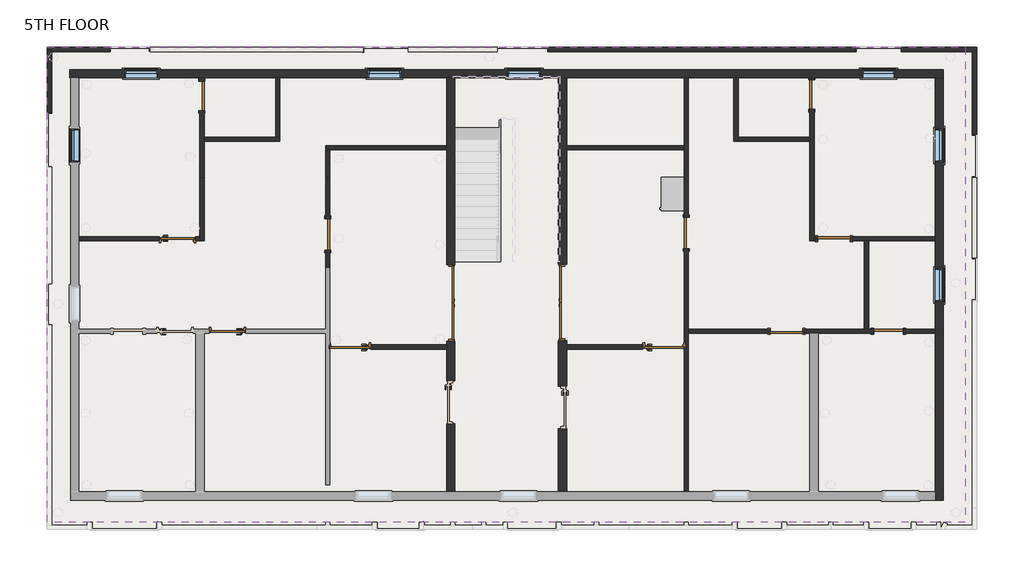
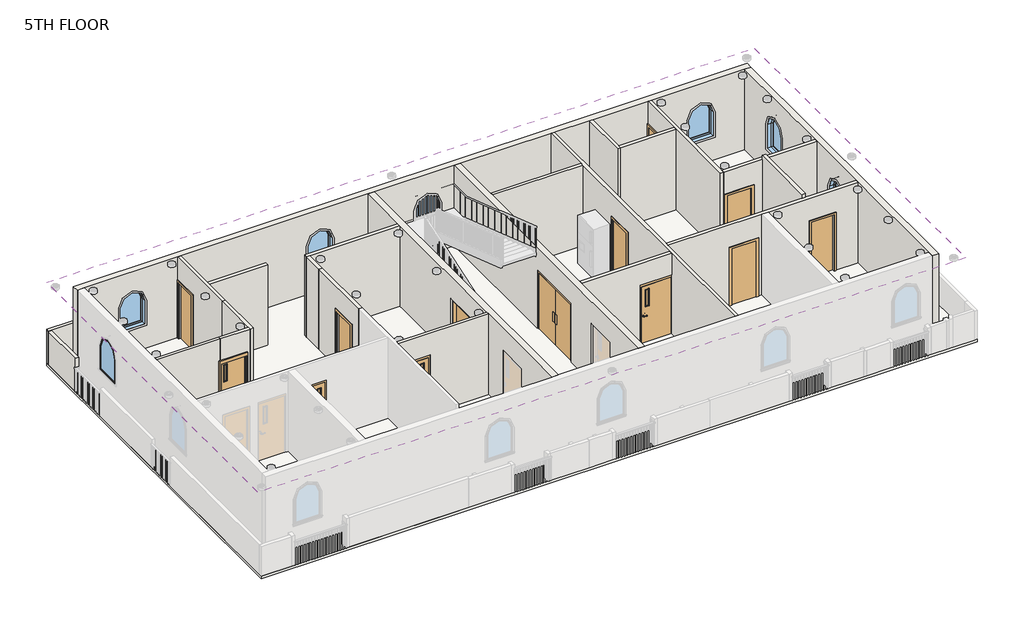
# One storey, part 2 of 7: 32 walls, 13 doors, 7 windows, 2 slabs, 1 covering.
"""IFC4 building model written with IfcOpenShell, lengths in millimetres."""

from ifc_helpers import new_model, si_unit, frame, origin, place, context, project, spatial, polyline, circle_curve, outline, extrude, faceted_brep, transform, mapped, element, save
from ifc_brep_helpers import plane_surface, revolved_surface, advanced_brep
from components import door_2c854dd0, door_cf1f2706, door_4f5842df, door_passage_single_vision_lite_3_x7_440dd290, door_70e57c00, door_700d3439, door_8cb1b8a7, door_38851409, door_d141acb4, window_fixed_round_top_3_x_4_dee2be1c

model = new_model("IFC4")

# Units and contexts
model_context = context("Model", 3, world=origin())
ifc_project = project(units=[si_unit("LENGTHUNIT", "METRE", prefix="MILLI")], contexts=[model_context])

# Site, building, storey
site = spatial("IfcSite", under=ifc_project)
building = spatial("IfcBuilding", under=site)
storey = spatial("IfcBuildingStorey", under=building, Name="5TH FLOOR", Elevation=16002.0)

# Covering
placement = place(None, origin())
element("IfcCovering", 1, ObjectType="2' x 4' ACT System", at=placement, inside=storey, context=model_context, shape_type="SweptSolid", body=[
    extrude(outline(polyline([(12235.5012075, 8470.0067329), (12235.5012075, -4623.6932193), (-13088.8067989, -4623.6932193), (-13088.8067989, 8470.0067329), (12235.5012075, 8470.0067329)])), frame((0.0, 0.0, 19050.0), z_axis=(0.0, 0.0, 1.0), x_axis=(1.0, 0.0, 0.0)), (0.0, 0.0, 1.0), 57.15),
])

# Doors
door_shape = door_2c854dd0(model_context)
element("IfcDoor", 2, ObjectType="Door-Passage-Double-Flush-Dbl_Acting : 6'79\" X 84\"", at=placement, inside=storey, context=model_context, shape_type="MappedRepresentation", body=[
    mapped(door_shape, transform((-1969.4487998, 1424.4578621, 16002.0), x_axis=(0.0, -1.0, 0.0), y_axis=(1.0, 0.0, 0.0), z_axis=(0.0, 0.0, 1.0))),
])
element("IfcDoor", 3, ObjectType="Door-Passage-Double-Flush-Dbl_Acting : 6'79\" X 84\"", at=placement, inside=storey, context=model_context, shape_type="MappedRepresentation", body=[
    mapped(door_shape, transform((1128.8432011, 1434.2067807, 16002.0), x_axis=(0.0, 1.0, 0.0), y_axis=(-1.0, 0.0, 0.0), z_axis=(0.0, 0.0, 1.0))),
])
door_2_shape = door_cf1f2706(model_context)
element("IfcDoor", 4, ObjectType="Door-Passage-Single-Vision_Lite : 3'6\"X7' 2", at=placement, inside=storey, context=model_context, shape_type="MappedRepresentation", body=[
    mapped(door_2_shape, transform((-4750.7487995, 211.6078621, 16002.0), x_axis=(-1.0, 0.0, 0.0), y_axis=(0.0, -1.0, 0.0), z_axis=(0.0, 0.0, 1.0))),
])
door_3_shape = door_4f5842df(model_context)
element("IfcDoor", 5, ObjectType="Door-Passage-Single-Vision_Lite : 3'6\"X7' 2", at=placement, inside=storey, context=model_context, shape_type="MappedRepresentation", body=[
    mapped(door_3_shape, transform((3923.3512082, 211.6078621, 16002.0), x_axis=(1.0, 0.0, 0.0), y_axis=(0.0, 1.0, 0.0), z_axis=(0.0, 0.0, 1.0))),
])
door_passage_single_vision_lite_3_x7_shape = door_passage_single_vision_lite_3_x7_440dd290(model_context)
element("IfcDoor", 6, ObjectType="Door-Passage-Single-Vision_Lite : 3'X7'", at=placement, inside=storey, context=model_context, shape_type="MappedRepresentation", body=[
    mapped(door_passage_single_vision_lite_3_x7_shape, transform((-9501.8462614, 3186.8067332, 16002.0), x_axis=(1.0, 0.0, 0.0), y_axis=(0.0, 1.0, 0.0), z_axis=(0.0, 0.0, 1.0))),
])
element("IfcDoor", 7, ObjectType="Door-Passage-Single-Vision_Lite : 3'X7'", at=placement, inside=storey, context=model_context, shape_type="MappedRepresentation", body=[
    mapped(door_passage_single_vision_lite_3_x7_shape, transform((-8122.5987992, 646.8067334, 16002.0), x_axis=(-1.0, 0.0, 0.0), y_axis=(0.0, -1.0, 0.0), z_axis=(0.0, 0.0, 1.0))),
])
door_4_shape = door_70e57c00(model_context)
element("IfcDoor", 8, ObjectType="Single-Flush : 2'10\" x 7'", at=placement, inside=storey, context=model_context, shape_type="MappedRepresentation", body=[
    mapped(door_4_shape, transform((-5360.3487995, 3313.8067802, 16002.0), x_axis=(0.0, -1.0, 0.0), y_axis=(1.0, 0.0, 0.0), z_axis=(0.0, 0.0, 1.0))),
])
door_5_shape = door_700d3439(model_context)
element("IfcDoor", 9, ObjectType="Single-Flush : 2'10\" x 7'", at=placement, inside=storey, context=model_context, shape_type="MappedRepresentation", body=[
    mapped(door_5_shape, transform((4532.9512082, 3351.906733, 16002.0), x_axis=(0.0, -1.0, 0.0), y_axis=(1.0, 0.0, 0.0), z_axis=(0.0, 0.0, 1.0))),
])
door_6_shape = door_8cb1b8a7(model_context)
element("IfcDoor", 10, ObjectType="Single-Flush : 2'11\"x 7'", at=placement, inside=storey, context=model_context, shape_type="MappedRepresentation", body=[
    mapped(door_6_shape, transform((8609.6512079, 3193.1567332, 16002.0), x_axis=(-1.0, 0.0, 0.0), y_axis=(0.0, -1.0, 0.0), z_axis=(0.0, 0.0, 1.0))),
])
element("IfcDoor", 11, ObjectType="Single-Flush : 2'11\"x 7'", at=placement, inside=storey, context=model_context, shape_type="MappedRepresentation", body=[
    mapped(door_6_shape, transform((7295.2012079, 640.4567334, 16002.0), x_axis=(1.0, 0.0, 0.0), y_axis=(0.0, 1.0, 0.0), z_axis=(0.0, 0.0, 1.0))),
])
door_7_shape = door_38851409(model_context)
element("IfcDoor", 12, ObjectType="Single-Flush : 2'8\"x 7'", at=placement, inside=storey, context=model_context, shape_type="MappedRepresentation", body=[
    mapped(door_7_shape, transform((-8827.4487992, 7136.5067329, 16002.0), x_axis=(0.0, 1.0, 0.0), y_axis=(-1.0, 0.0, 0.0), z_axis=(0.0, 0.0, 1.0))),
])
element("IfcDoor", 13, ObjectType="Single-Flush : 2'8\"x 7'", at=placement, inside=storey, context=model_context, shape_type="MappedRepresentation", body=[
    mapped(door_7_shape, transform((10111.5098918, 640.4567334, 16002.0), x_axis=(-1.0, 0.0, 0.0), y_axis=(0.0, -1.0, 0.0), z_axis=(0.0, 0.0, 1.0))),
])
door_8_shape = door_d141acb4(model_context)
element("IfcDoor", 14, ObjectType="Single-Flush : 2'8\"x 7'", at=placement, inside=storey, context=model_context, shape_type="MappedRepresentation", body=[
    mapped(door_8_shape, transform((8000.0512079, 7167.840939, 16002.0), x_axis=(0.0, 1.0, 0.0), y_axis=(-1.0, 0.0, 0.0), z_axis=(0.0, 0.0, 1.0))),
])

# Slabs
element("IfcSlab", 15, ObjectType="LW Concrete on Metal Deck", at=placement, inside=storey, context=model_context, shape_type="SweptSolid", body=[
    extrude(outline(polyline([(12540.3012043, 8470.0067329), (12540.3012043, -4826.8932661), (-13088.8067989, -4826.8932661), (-13088.8067989, 8470.0067329), (12540.3012043, 8470.0067329)])), frame((0.0, 0.0, 15897.225), z_axis=(0.0, 0.0, 1.0), x_axis=(1.0, 0.0, 0.0)), (0.0, 0.0, 1.0), 104.775),
])
element("IfcSlab", 16, ObjectType="LW Concrete on Metal Deck", at=placement, inside=storey, context=model_context, shape_type="SweptSolid", body=[
    extrude(outline(polyline([(12540.3012043, 8470.0067329), (12540.3012043, -4826.8932661), (-13088.8067989, -4826.8932661), (-13088.8067989, 8470.0067329), (12540.3012043, 8470.0067329)])), frame((0.0, 0.0, 15897.225), z_axis=(0.0, 0.0, 1.0), x_axis=(1.0, 0.0, 0.0)), (0.0, 0.0, 1.0), 104.775),
])

# Walls
element("IfcWall", 17, ObjectType="Generic - 4.5\"", at=placement, inside=storey, context=model_context, shape_type="SweptSolid", body=[
    extrude(outline(polyline([(19050.0, -9959.0462614), (19050.0, -12224.6987925), (16002.0, -12224.6987925), (16002.0, -10009.8462614), (18237.2, -10009.8462614), (18237.2, -9959.0462614), (19050.0, -9959.0462614)])), frame((0.0, 3136.0067332, 0.0), z_axis=(0.0, 1.0, 0.0), x_axis=(0.0, 0.0, 1.0)), (0.0, 0.0, 1.0), 114.3),
])
element("IfcWall", 18, ObjectType="Generic - 4.5\"", at=placement, inside=storey, context=model_context, shape_type="Brep", body=[
    faceted_brep([(-8884.5987992, 4875.906733, 16002.0), (-8884.5987992, 3250.3067332, 16002.0), (-8884.5987992, 3136.0067332, 16002.0), (-8884.5987992, 3136.0067332, 19050.0), (-8884.5987992, 3250.3067332, 19050.0), (-8884.5987992, 4875.906733, 19050.0), (-8770.2987992, 4875.906733, 16002.0), (-8770.2987992, 4875.906733, 19050.0), (-8770.2987992, 3136.0067332, 19050.0), (-8770.2987992, 3136.0067332, 16002.0)], [[[0, 1, 2, 3, 4, 5]], [[6, 7, 8, 9]], [[2, 1, 0, 6, 9]], [[5, 4, 3, 8, 7]], [[0, 5, 7, 6]], [[3, 2, 9, 8]]]),
])
element("IfcWall", 19, ObjectType="Generic - 4.5\"", at=placement, inside=storey, context=model_context, shape_type="SweptSolid", body=[
    extrude(outline(polyline([(19050.0, -2077.3987998), (19050.0, -5303.1987995), (18237.2, -5303.1987995), (18237.2, -4166.5487995), (16002.0, -4166.5487995), (16002.0, -2077.3987998), (19050.0, -2077.3987998)])), frame((0.0, 148.1078621, 0.0), z_axis=(0.0, 1.0, 0.0), x_axis=(0.0, 0.0, 1.0)), (0.0, 0.0, 1.0), 114.3),
])
element("IfcWall", 20, ObjectType="Generic - 4.5\"", at=placement, inside=storey, context=model_context, shape_type="Brep", body=[
    faceted_brep([(-2077.3987998, 5764.9067329, 16002.0), (-5417.4987995, 5764.9067329, 16002.0), (-5417.4987995, 5764.9067329, 19050.0), (-2077.3987998, 5764.9067329, 19050.0), (-2077.3987998, 5650.6067329, 16002.0), (-2077.3987998, 5650.6067329, 19050.0), (-5303.1987995, 5650.6067329, 19050.0), (-5417.4987995, 5650.6067329, 19050.0), (-5417.4987995, 5650.6067329, 16002.0), (-5303.1987995, 5650.6067329, 16002.0)], [[[0, 1, 2, 3]], [[4, 5, 6, 7, 8, 9]], [[1, 0, 4, 9, 8]], [[3, 2, 7, 6, 5]], [[2, 1, 8, 7]], [[0, 3, 5, 4]]]),
])
element("IfcWall", 21, ObjectType="Generic - 4.5\"", at=placement, inside=storey, context=model_context, shape_type="SweptSolid", body=[
    extrude(outline(polyline([(-5417.4987995, 4875.90678), (-5417.4987995, 5650.6067329), (-5303.1987995, 5650.6067329), (-5303.1987995, 4875.90678), (-5417.4987995, 4875.90678)])), frame((0.0, 0.0, 16002.0), z_axis=(0.0, 0.0, 1.0), x_axis=(1.0, 0.0, 0.0)), (0.0, 0.0, 1.0), 3048.0),
])
element("IfcWall", 22, ObjectType="Generic - 4.5\"", at=placement, inside=storey, context=model_context, shape_type="SweptSolid", body=[
    extrude(outline(polyline([(4475.8012082, 5650.6067329), (1250.0012085, 5650.6067329), (1250.0012085, 5764.9067329), (4475.8012082, 5764.9067329), (4475.8012082, 5650.6067329)])), frame((0.0, 0.0, 16002.0), z_axis=(0.0, 0.0, 1.0), x_axis=(1.0, 0.0, 0.0)), (0.0, 0.0, 1.0), 3048.0),
])
element("IfcWall", 23, ObjectType="Generic - 4.5\"", at=placement, inside=storey, context=model_context, shape_type="Brep", body=[
    faceted_brep([(4475.8012082, -3785.4932193, 19050.0), (4475.8012082, 148.1078621, 19050.0), (4475.8012082, 262.4078621, 19050.0), (4475.8012082, 5650.6067329, 19050.0), (4475.8012082, 5764.9067329, 19050.0), (4475.8012082, 7631.8067329, 19050.0), (4475.8012082, 7631.8067329, 16002.0), (4475.8012082, 5764.9067329, 16002.0), (4475.8012082, 5650.6067329, 16002.0), (4475.8012082, 3783.706733, 16002.0), (4475.8012082, 3783.706733, 18135.6), (4475.8012082, 2920.106733, 18135.6), (4475.8012082, 2920.106733, 16002.0), (4475.8012082, 262.4078621, 16002.0), (4475.8012082, 262.4078621, 18237.2), (4475.8012082, 148.1078621, 18237.2), (4475.8012082, 148.1078621, 16002.0), (4475.8012082, -3785.4932193, 16002.0), (4590.1012082, 7631.8067329, 19050.0), (4590.1012082, 697.6067334, 19050.0), (4590.1012082, 583.3067334, 19050.0), (4590.1012082, -3785.4932193, 19050.0), (4590.1012082, -3785.4932193, 16002.0), (4590.1012082, 583.3067334, 16002.0), (4590.1012082, 697.6067334, 16002.0), (4590.1012082, 2920.106733, 16002.0), (4590.1012082, 2920.106733, 18135.6), (4590.1012082, 3783.706733, 18135.6), (4590.1012082, 3783.706733, 16002.0), (4590.1012082, 7631.8067329, 16002.0), (4507.5512082, 148.1078621, 16002.0), (4507.5512082, 262.4078621, 16002.0), (4507.5512082, 148.1078621, 18237.2), (4507.5512082, 262.4078621, 18237.2)], [[[0, 1, 2, 3, 4, 5, 6, 7, 8, 9, 10, 11, 12, 13, 14, 15, 16, 17]], [[18, 19, 20, 21, 22, 23, 24, 25, 26, 27, 28, 29]], [[6, 29, 28, 9, 8, 7]], [[12, 25, 24, 23, 22, 17, 16, 30, 31, 13]], [[5, 4, 3, 2, 1, 0, 21, 20, 19, 18]], [[6, 5, 18, 29]], [[28, 27, 10, 9]], [[27, 26, 11, 10]], [[26, 25, 12, 11]], [[0, 17, 22, 21]], [[32, 30, 16, 15]], [[31, 33, 14, 13]], [[30, 32, 33, 31]], [[33, 32, 15, 14]]]),
])
element("IfcWall", 24, ObjectType="Generic - 4.5\"", at=placement, inside=storey, context=model_context, shape_type="Brep", body=[
    faceted_brep([(5847.401208, 7631.8067329, 16002.0), (5847.401208, 5879.2067329, 16002.0), (5847.401208, 5879.2067329, 19050.0), (5847.401208, 7631.8067329, 19050.0), (5961.701208, 7631.8067329, 16002.0), (5961.701208, 7631.8067329, 19050.0), (5961.701208, 5993.5067329, 19050.0), (5961.701208, 5879.2067329, 19050.0), (5961.701208, 5879.2067329, 16002.0), (5961.701208, 5993.5067329, 16002.0)], [[[0, 1, 2, 3]], [[4, 5, 6, 7, 8, 9]], [[1, 0, 4, 9, 8]], [[3, 2, 7, 6, 5]], [[0, 3, 5, 4]], [[2, 1, 8, 7]]]),
])
element("IfcWall", 25, ObjectType="Generic - 4.5\"", at=placement, inside=storey, context=model_context, shape_type="SweptSolid", body=[
    extrude(outline(polyline([(7942.9012079, 5879.2067329), (5961.701208, 5879.2067329), (5961.701208, 5993.5067329), (7942.9012079, 5993.5067329), (7942.9012079, 5879.2067329)])), frame((0.0, 0.0, 16002.0), z_axis=(0.0, 0.0, 1.0), x_axis=(1.0, 0.0, 0.0)), (0.0, 0.0, 1.0), 3048.0),
])
element("IfcWall", 26, ObjectType="Generic - 4.5\"", at=placement, inside=storey, context=model_context, shape_type="Brep", body=[
    faceted_brep([(7942.9012079, 7625.040939, 16002.0), (7942.9012079, 7574.240939, 16002.0), (7942.9012079, 7574.240939, 18135.6), (7942.9012079, 6761.440939, 18135.6), (7942.9012079, 6761.440939, 16002.0), (7942.9012079, 5993.5067329, 16002.0), (7942.9012079, 5879.2067329, 16002.0), (7942.9012079, 3136.0067332, 16002.0), (7942.9012079, 3136.0067332, 19050.0), (7942.9012079, 5879.2067329, 19050.0), (7942.9012079, 5993.5067329, 19050.0), (7942.9012079, 7625.040939, 19050.0), (8057.2012079, 7574.240939, 18135.6), (8057.2012079, 7574.240939, 16002.0), (8057.2012079, 7625.040939, 16002.0), (8057.2012079, 7625.040939, 19050.0), (8057.2012079, 3250.3067332, 19050.0), (8057.2012079, 3136.0067332, 19050.0), (8057.2012079, 3136.0067332, 16002.0), (8057.2012079, 3250.3067332, 16002.0), (8057.2012079, 6761.440939, 16002.0), (8057.2012079, 6761.440939, 18135.6)], [[[0, 1, 2, 3, 4, 5, 6, 7, 8, 9, 10, 11]], [[12, 13, 14, 15, 16, 17, 18, 19, 20, 21]], [[14, 13, 1, 0]], [[20, 19, 18, 7, 6, 5, 4]], [[11, 10, 9, 8, 17, 16, 15]], [[0, 11, 15, 14]], [[8, 7, 18, 17]], [[2, 1, 13, 12]], [[3, 2, 12, 21]], [[4, 3, 21, 20]]]),
])
element("IfcWall", 27, ObjectType="Generic - 4.5\"", at=placement, inside=storey, context=model_context, shape_type="Brep", body=[
    faceted_brep([(8165.1512079, 3250.3067332, 18135.6), (8165.1512079, 3250.3067332, 16002.0), (8057.2012079, 3250.3067332, 16002.0), (8057.2012079, 3250.3067332, 19050.0), (11397.3012075, 3250.3067332, 19050.0), (11397.3012075, 3250.3067332, 16002.0), (9054.1512079, 3250.3067332, 16002.0), (9054.1512079, 3250.3067332, 18135.6), (8057.2012079, 3136.0067332, 16002.0), (8165.1512079, 3136.0067332, 16002.0), (8165.1512079, 3136.0067332, 18135.6), (9054.1512079, 3136.0067332, 18135.6), (9054.1512079, 3136.0067332, 16002.0), (9438.4098918, 3136.0067332, 16002.0), (9565.4098918, 3136.0067332, 16002.0), (11397.3012075, 3136.0067332, 16002.0), (11397.3012075, 3136.0067332, 19050.0), (8057.2012079, 3136.0067332, 19050.0)], [[[0, 1, 2, 3, 4, 5, 6, 7]], [[8, 9, 10, 11, 12, 13, 14, 15, 16, 17]], [[6, 5, 15, 14, 13, 12]], [[2, 1, 9, 8]], [[4, 3, 17, 16]], [[3, 2, 8, 17]], [[5, 4, 16, 15]], [[10, 9, 1, 0]], [[11, 10, 0, 7]], [[12, 11, 7, 6]]]),
])
element("IfcWall", 28, ObjectType="Generic - 4.5\"", at=placement, inside=storey, context=model_context, shape_type="Brep", body=[
    faceted_brep([(7739.7012079, 583.3067334, 18135.6), (7739.7012079, 583.3067334, 16002.0), (7942.9012079, 583.3067334, 16002.0), (8171.5012079, 583.3067334, 16002.0), (9705.1098918, 583.3067334, 16002.0), (9705.1098918, 583.3067334, 18135.6), (10517.9098918, 583.3067334, 18135.6), (10517.9098918, 583.3067334, 16002.0), (11397.3012075, 583.3067334, 16002.0), (11397.3012075, 583.3067334, 19050.0), (8171.5012079, 583.3067334, 19050.0), (7942.9012079, 583.3067334, 19050.0), (4590.1012082, 583.3067334, 19050.0), (4590.1012082, 583.3067334, 16002.0), (6850.7012079, 583.3067334, 16002.0), (6850.7012079, 583.3067334, 18135.6), (9705.1098918, 697.6067334, 16002.0), (9565.4098918, 697.6067334, 16002.0), (9438.4098918, 697.6067334, 16002.0), (7739.7012079, 697.6067334, 16002.0), (7739.7012079, 697.6067334, 18135.6), (6850.7012079, 697.6067334, 18135.6), (6850.7012079, 697.6067334, 16002.0), (4590.1012082, 697.6067334, 16002.0), (4590.1012082, 697.6067334, 19050.0), (11397.3012075, 697.6067334, 19050.0), (11397.3012075, 697.6067334, 16002.0), (10517.9098918, 697.6067334, 16002.0), (10517.9098918, 697.6067334, 18135.6), (9705.1098918, 697.6067334, 18135.6)], [[[0, 1, 2, 3, 4, 5, 6, 7, 8, 9, 10, 11, 12, 13, 14, 15]], [[16, 17, 18, 19, 20, 21, 22, 23, 24, 25, 26, 27, 28, 29]], [[27, 26, 8, 7]], [[14, 13, 23, 22]], [[4, 3, 2, 1, 19, 18, 17, 16]], [[12, 11, 10, 9, 25, 24]], [[9, 8, 26, 25]], [[13, 12, 24, 23]], [[5, 4, 16, 29]], [[6, 5, 29, 28]], [[7, 6, 28, 27]], [[20, 19, 1, 0]], [[21, 20, 0, 15]], [[22, 21, 15, 14]]]),
])
element("IfcWall", 29, ObjectType="Generic - 4.5\"", at=placement, inside=storey, context=model_context, shape_type="Brep", body=[
    faceted_brep([(-8770.2987992, 7542.9067329, 18135.6), (-8770.2987992, 7542.9067329, 16002.0), (-8770.2987992, 7631.8067329, 16002.0), (-8770.2987992, 7631.8067329, 19050.0), (-8770.2987992, 5993.5067329, 19050.0), (-8770.2987992, 5879.2067329, 19050.0), (-8770.2987992, 4875.906733, 19050.0), (-8770.2987992, 4875.906733, 16002.0), (-8770.2987992, 5879.2067329, 16002.0), (-8770.2987992, 5993.5067329, 16002.0), (-8770.2987992, 6730.1067329, 16002.0), (-8770.2987992, 6730.1067329, 18135.6), (-8884.5987992, 7631.8067329, 16002.0), (-8884.5987992, 7542.9067329, 16002.0), (-8884.5987992, 7542.9067329, 18135.6), (-8884.5987992, 6730.1067329, 18135.6), (-8884.5987992, 6730.1067329, 16002.0), (-8884.5987992, 4875.906733, 16002.0), (-8884.5987992, 4875.906733, 19050.0), (-8884.5987992, 7631.8067329, 19050.0)], [[[0, 1, 2, 3, 4, 5, 6, 7, 8, 9, 10, 11]], [[12, 13, 14, 15, 16, 17, 18, 19]], [[2, 1, 13, 12]], [[10, 9, 8, 7, 17, 16]], [[6, 5, 4, 3, 19, 18]], [[7, 6, 18, 17]], [[3, 2, 12, 19]], [[14, 13, 1, 0]], [[15, 14, 0, 11]], [[16, 15, 11, 10]]]),
])
element("IfcWall", 30, ObjectType="Generic - 4.5\"", at=placement, inside=storey, context=model_context, shape_type="Brep", body=[
    faceted_brep([(-8770.2987992, 5879.2067329, 16002.0), (-6674.7987994, 5879.2067329, 16002.0), (-6674.7987994, 5879.2067329, 19050.0), (-8770.2987992, 5879.2067329, 19050.0), (-8770.2987992, 5993.5067329, 16002.0), (-8770.2987992, 5993.5067329, 19050.0), (-6674.7987994, 5993.5067329, 19050.0), (-6674.7987994, 5993.5067329, 17373.6), (-6674.7987994, 5993.5067329, 16002.0), (-6789.0987994, 5993.5067329, 16002.0)], [[[0, 1, 2, 3]], [[4, 5, 6, 7, 8, 9]], [[1, 0, 4, 9, 8]], [[3, 2, 6, 5]], [[0, 3, 5, 4]], [[2, 1, 8, 7, 6]]]),
])
element("IfcWall", 31, ObjectType="Generic - 4.5\"", at=placement, inside=storey, context=model_context, shape_type="SweptSolid", body=[
    extrude(outline(polyline([(-6674.7987994, 7631.8067329), (-6674.7987994, 5993.5067329), (-6789.0987994, 5993.5067329), (-6789.0987994, 7631.8067329), (-6674.7987994, 7631.8067329)])), frame((0.0, 0.0, 16002.0), z_axis=(0.0, 0.0, 1.0), x_axis=(1.0, 0.0, 0.0)), (0.0, 0.0, 1.0), 1371.6),
])
element("IfcWall", 32, ObjectType="Generic - 4.5\"", at=placement, inside=storey, context=model_context, shape_type="SweptSolid", body=[
    extrude(outline(polyline([(19050.0, -8884.5987992), (19050.0, -9959.0462614), (18237.2, -9959.0462614), (18237.2, -8993.8462614), (16002.0, -8993.8462614), (16002.0, -8884.5987992), (19050.0, -8884.5987992)])), frame((0.0, 3136.0067332, 0.0), z_axis=(0.0, 1.0, 0.0), x_axis=(0.0, 0.0, 1.0)), (0.0, 0.0, 1.0), 114.3),
])
element("IfcWall", 33, ObjectType="Generic - 4.5\"", at=placement, inside=storey, context=model_context, shape_type="SweptSolid", body=[
    extrude(outline(polyline([(2882.0067802, 18135.6), (2882.0067802, 16002.0), (2399.4067802, 16002.0), (2399.4067802, 19050.0), (4875.90678, 19050.0), (4875.90678, 16002.0), (3745.6067802, 16002.0), (3745.6067802, 18135.6), (2882.0067802, 18135.6)])), frame((-5417.4987995, 0.0, 0.0), z_axis=(1.0, 0.0, 0.0), x_axis=(0.0, 1.0, 0.0)), (0.0, 0.0, 1.0), 114.3),
])
element("IfcWall", 34, ObjectType="Generic - 4.5\"", at=placement, inside=storey, context=model_context, shape_type="SweptSolid", body=[
    extrude(outline(polyline([(19050.0, 4475.8012082), (19050.0, 1250.0012085), (16002.0, 1250.0012085), (16002.0, 3339.1512082), (18237.2, 3339.1512082), (18237.2, 4475.8012082), (19050.0, 4475.8012082)])), frame((0.0, 148.1078621, 0.0), z_axis=(0.0, 1.0, 0.0), x_axis=(0.0, 0.0, 1.0)), (0.0, 0.0, 1.0), 114.3),
])
element("IfcWall", 35, ObjectType="Generic - 4.5\"", at=placement, inside=storey, context=model_context, shape_type="SweptSolid", body=[
    extrude(outline(polyline([(-12973.9987925, 8412.8567329), (-12973.9987925, 6682.2711337), (-13088.2987925, 6682.2711337), (-13088.2987925, 8412.8567329), (-12973.9987925, 8412.8567329)])), frame((0.0, 0.0, 16002.0), z_axis=(0.0, 0.0, 1.0), x_axis=(1.0, 0.0, 0.0)), (0.0, 0.0, 1.0), 1259.0059812),
])
element("IfcWall", 36, ObjectType="Generic - 4.5\"", at=placement, inside=storey, context=model_context, shape_type="SweptSolid", body=[
    extrude(outline(polyline([(-11387.0067989, 8355.7067329), (-13088.8067989, 8355.7067329), (-13088.8067989, 8470.0067329), (-11387.0067989, 8470.0067329), (-11387.0067989, 8355.7067329)])), frame((0.0, 0.0, 16002.0), z_axis=(0.0, 0.0, 1.0), x_axis=(1.0, 0.0, 0.0)), (0.0, 0.0, 1.0), 1273.4134002),
])
element("IfcWall", 37, ObjectType="Generic - 4.5\"", at=placement, inside=storey, context=model_context, shape_type="SweptSolid", body=[
    extrude(outline(polyline([(-4382.4487992, 8355.7067329), (-10247.1817989, 8355.7067329), (-10247.1817989, 8470.0067329), (-4382.4487992, 8470.0067329), (-4382.4487992, 8355.7067329)])), frame((0.0, 0.0, 16002.0), z_axis=(0.0, 0.0, 1.0), x_axis=(1.0, 0.0, 0.0)), (0.0, 0.0, 1.0), 1083.89837),
])
element("IfcWall", 38, ObjectType="Generic - 4.5\"", at=placement, inside=storey, context=model_context, shape_type="SweptSolid", body=[
    extrude(outline(polyline([(-682.0490672, 8355.7067329), (-3139.4990672, 8355.7067329), (-3139.4990672, 8470.0067329), (-682.0490672, 8470.0067329), (-682.0490672, 8355.7067329)])), frame((0.0, 0.0, 16002.0), z_axis=(0.0, 0.0, 1.0), x_axis=(1.0, 0.0, 0.0)), (0.0, 0.0, 1.0), 1195.9732529),
])
element("IfcWall", 39, ObjectType="Generic - 4.5\"", at=placement, inside=storey, context=model_context, shape_type="SweptSolid", body=[
    extrude(outline(polyline([(9199.6932011, 8355.7067329), (741.4932011, 8355.7067329), (741.4932011, 8470.0067329), (9199.6932011, 8470.0067329), (9199.6932011, 8355.7067329)])), frame((0.0, 0.0, 16002.0), z_axis=(0.0, 0.0, 1.0), x_axis=(1.0, 0.0, 0.0)), (0.0, 0.0, 1.0), 1274.1868366),
])
element("IfcWall", 40, ObjectType="Generic - 4.5\"", at=placement, inside=storey, context=model_context, shape_type="Brep", body=[
    faceted_brep([(10462.2009401, 8355.7067329, 16002.0), (12426.0012043, 8355.7067329, 16002.0), (12540.3012043, 8355.7067329, 16002.0), (12540.3012043, 8355.7067329, 17367.7502881), (10462.2009401, 8355.7067329, 17367.7502881), (10462.2009401, 8470.0067329, 16002.0), (10462.2009401, 8470.0067329, 17367.7502881), (12540.3012043, 8470.0067329, 17367.7502881), (12540.3012043, 8470.0067329, 16002.0)], [[[0, 1, 2, 3, 4]], [[5, 6, 7, 8]], [[2, 1, 0, 5, 8]], [[4, 3, 7, 6]], [[0, 4, 6, 5]], [[3, 2, 8, 7]]]),
])
element("IfcWall", 41, ObjectType="Generic - 4.5\"", at=placement, inside=storey, context=model_context, shape_type="Brep", body=[
    faceted_brep([(12426.0012043, 8355.7067329, 16002.0), (12426.0012043, 6069.7067329, 16002.0), (12426.0012043, 6069.7067329, 17373.6), (12426.0012043, 8355.7067329, 17373.6), (12540.3012043, 8355.7067329, 16002.0), (12540.3012043, 8355.7067329, 17367.7502881), (12540.3012043, 8355.7067329, 17373.6), (12540.3012043, 6069.7067329, 17373.6), (12540.3012043, 6069.7067329, 16002.0)], [[[0, 1, 2, 3]], [[4, 5, 6, 7, 8]], [[1, 0, 4, 8]], [[2, 1, 8, 7]], [[3, 2, 7, 6]], [[0, 3, 6, 5, 4]]]),
])
element("IfcWall", 42, ObjectType="Generic - 4.5\"", at=placement, inside=storey, context=model_context, shape_type="SweptSolid", body=[
    extrude(outline(polyline([(12426.0012043, 2666.1067329), (12426.0012043, 4875.9067329), (12540.3012043, 4875.9067329), (12540.3012043, 2666.1067329), (12426.0012043, 2666.1067329)])), frame((0.0, 0.0, 16002.0), z_axis=(0.0, 0.0, 1.0), x_axis=(1.0, 0.0, 0.0)), (0.0, 0.0, 1.0), 1193.0409005),
])
element("IfcWall", 43, ObjectType="Generic - 9\"", at=placement, inside=storey, context=model_context, shape_type="AdvancedBrep", body=[
    advanced_brep(
    [(-12479.2067989, 7631.8067329, 16002.0), (-12453.2987925, 7631.8067329, 16002.0), (-12224.6987925, 7631.8067329, 16002.0), (-8884.5987992, 7631.8067329, 16002.0), (-8770.2987992, 7631.8067329, 16002.0), (-6789.0987994, 7631.8067329, 16002.0), (-6674.7987994, 7631.8067329, 16002.0), (-2077.3987998, 7631.8067329, 16002.0), (-1848.7987998, 7631.8067329, 16002.0), (1008.1932011, 7631.8067329, 16002.0), (1236.7932011, 7631.8067329, 16002.0), (4475.8012082, 7631.8067329, 16002.0), (4590.1012082, 7631.8067329, 16002.0), (5847.401208, 7631.8067329, 16002.0), (5961.701208, 7631.8067329, 16002.0), (11397.3012075, 7631.8067329, 16002.0), (11625.9012075, 7631.8067329, 16002.0), (11625.9012075, 7631.8067329, 19050.0), (11397.3012075, 7631.8067329, 19050.0), (5961.701208, 7631.8067329, 19050.0), (5847.401208, 7631.8067329, 19050.0), (4590.1012082, 7631.8067329, 19050.0), (4475.8012082, 7631.8067329, 19050.0), (1236.7932011, 7631.8067329, 19050.0), (1008.1932011, 7631.8067329, 19050.0), (-1848.7987998, 7631.8067329, 19050.0), (-2077.3987998, 7631.8067329, 19050.0), (-8770.2987992, 7631.8067329, 19050.0), (-8884.5987992, 7631.8067329, 19050.0), (-12224.6987925, 7631.8067329, 19050.0), (-12453.2987925, 7631.8067329, 19050.0), (-12479.2067989, 7631.8067329, 19050.0), (9378.0012075, 7631.8067329, 16916.4), (9378.0012075, 7631.8067329, 17830.8), (10292.4012075, 7631.8067329, 17830.8), (10292.4012075, 7631.8067329, 16916.4), (-401.5067989, 7631.8067329, 16916.4), (-401.5067989, 7631.8067329, 17830.8), (512.8932011, 7631.8067329, 17830.8), (512.8932011, 7631.8067329, 16916.4), (-4249.0987998, 7631.8067329, 16916.4), (-4249.0987998, 7631.8067329, 17830.8), (-3334.6987998, 7631.8067329, 17830.8), (-3334.6987998, 7631.8067329, 16916.4), (-10961.0487992, 7631.8067329, 16916.4), (-10961.0487992, 7631.8067329, 17830.8), (-10046.6487992, 7631.8067329, 17830.8), (-10046.6487992, 7631.8067329, 16916.4), (-12479.2067989, 7860.4067329, 16002.0), (-12479.2067989, 7860.4067329, 19050.0), (11625.9012075, 7860.4067329, 19050.0), (11625.9012075, 7860.4067329, 16002.0), (9378.0012075, 7860.4067329, 16916.4), (10292.4012075, 7860.4067329, 16916.4), (10292.4012075, 7860.4067329, 17830.8), (9378.0012075, 7860.4067329, 17830.8), (-401.5067989, 7860.4067329, 16916.4), (512.8932011, 7860.4067329, 16916.4), (512.8932011, 7860.4067329, 17830.8), (-401.5067989, 7860.4067329, 17830.8), (-4249.0987998, 7860.4067329, 16916.4), (-3334.6987998, 7860.4067329, 16916.4), (-3334.6987998, 7860.4067329, 17830.8), (-4249.0987998, 7860.4067329, 17830.8), (-10961.0487992, 7860.4067329, 16916.4), (-10046.6487992, 7860.4067329, 16916.4), (-10046.6487992, 7860.4067329, 17830.8), (-10961.0487992, 7860.4067329, 17830.8)],
    [
        (0, 1),
        (1, 2),
        (2, 3),
        (3, 4),
        (4, 5),
        (5, 6),
        (6, 7),
        (7, 8),
        (8, 9),
        (9, 10),
        (10, 11),
        (11, 12),
        (12, 13),
        (13, 14),
        (14, 15),
        (15, 16),
        (16, 17),
        (17, 18),
        (18, 19),
        (19, 20),
        (20, 21),
        (21, 22),
        (22, 23),
        (23, 24),
        (24, 25),
        (25, 26),
        (26, 27),
        (27, 28),
        (28, 29),
        (29, 30),
        (30, 31),
        (31, 0),
        (32, 33),
        (33, 34, circle_curve(frame((9835.2012075, 7631.8067329, 17830.8), z_axis=(0.0, 1.0, 0.0), x_axis=(1.0, 0.0, 0.0)), 457.2)),
        (34, 35),
        (35, 32),
        (36, 37),
        (37, 38, circle_curve(frame((55.6932011, 7631.8067329, 17830.8), z_axis=(0.0, 1.0, 0.0), x_axis=(1.0, 0.0, 0.0)), 457.2)),
        (38, 39),
        (39, 36),
        (40, 41),
        (41, 42, circle_curve(frame((-3791.8987998, 7631.8067329, 17830.8), z_axis=(0.0, 1.0, 0.0), x_axis=(1.0, 0.0, 0.0)), 457.2)),
        (42, 43),
        (43, 40),
        (44, 45),
        (45, 46, circle_curve(frame((-10503.8487992, 7631.8067329, 17830.8), z_axis=(0.0, 1.0, 0.0), x_axis=(1.0, 0.0, 0.0)), 457.2)),
        (46, 47),
        (47, 44),
        (48, 49),
        (49, 50),
        (50, 51),
        (51, 48),
        (52, 53),
        (53, 54),
        (54, 55, circle_curve(frame((9835.2012075, 7860.4067329, 17830.8), z_axis=(0.0, -1.0, 0.0), x_axis=(1.0, 0.0, 0.0)), 457.2)),
        (55, 52),
        (56, 57),
        (57, 58),
        (58, 59, circle_curve(frame((55.6932011, 7860.4067329, 17830.8), z_axis=(0.0, -1.0, 0.0), x_axis=(1.0, 0.0, 0.0)), 457.2)),
        (59, 56),
        (60, 61),
        (61, 62),
        (62, 63, circle_curve(frame((-3791.8987998, 7860.4067329, 17830.8), z_axis=(0.0, -1.0, 0.0), x_axis=(1.0, 0.0, 0.0)), 457.2)),
        (63, 60),
        (64, 65),
        (65, 66),
        (66, 67, circle_curve(frame((-10503.8487992, 7860.4067329, 17830.8), z_axis=(0.0, -1.0, 0.0), x_axis=(1.0, 0.0, 0.0)), 457.2)),
        (67, 64),
        (0, 48),
        (51, 16),
        (17, 50),
        (49, 31),
        (52, 32),
        (35, 53),
        (34, 54),
        (33, 55),
        (56, 36),
        (39, 57),
        (38, 58),
        (37, 59),
        (60, 40),
        (43, 61),
        (42, 62),
        (41, 63),
        (64, 44),
        (47, 65),
        (46, 66),
        (45, 67),
    ],
    [
        plane_surface(frame((-12479.2067989, 7631.8067329, 16002.0), z_axis=(0.0, -1.0, 0.0), x_axis=(1.0, 0.0, 0.0))),
        plane_surface(frame((-12479.2067989, 7860.4067329, 16002.0), z_axis=(0.0, 1.0, 0.0), x_axis=(-1.0, 0.0, 0.0))),
        plane_surface(frame((-12479.2067989, 7631.8067329, 16002.0), z_axis=(0.0, 0.0, -1.0), x_axis=(0.0, 1.0, 0.0))),
        plane_surface(frame((11511.6012075, 7631.8067329, 19050.0), z_axis=(0.0, 0.0, 1.0), x_axis=(0.0, 1.0, 0.0))),
        plane_surface(frame((-12479.2067989, 7631.8067329, 19050.0), z_axis=(-1.0, 0.0, 0.0), x_axis=(0.0, 1.0, 0.0))),
        plane_surface(frame((11625.9012075, 7629.6366753, 16002.0), z_axis=(1.0, 0.0, 0.0), x_axis=(0.0, 1.0, 0.0))),
        plane_surface(frame((9378.0012075, 7860.4067329, 16916.4), z_axis=(0.0, 0.0, 1.0), x_axis=(0.0, -1.0, 0.0))),
        plane_surface(frame((10292.4012075, 7860.4067329, 16916.4), z_axis=(-1.0, 0.0, 0.0), x_axis=(0.0, -1.0, 0.0))),
        revolved_surface(polyline([(10292.401207500001, 7631.8067329, 17830.8), (10292.401207500001, 7860.4067329, 17830.8)]), (9835.2012075, 7631.8067329, 17830.8), (0.0, -1.0, 0.0)),
        plane_surface(frame((9378.0012075, 7860.4067329, 17830.8), z_axis=(1.0, 0.0, 0.0), x_axis=(0.0, -1.0, 0.0))),
        plane_surface(frame((-401.5067989, 7860.4067329, 16916.4), z_axis=(0.0, 0.0, 1.0), x_axis=(0.0, -1.0, 0.0))),
        plane_surface(frame((512.8932011, 7860.4067329, 16916.4), z_axis=(-1.0, 0.0, 0.0), x_axis=(0.0, -1.0, 0.0))),
        revolved_surface(polyline([(512.8932010999999, 7631.8067329, 17830.8), (512.8932010999999, 7860.4067329, 17830.8)]), (55.6932011, 7631.8067329, 17830.8), (0.0, -1.0, 0.0)),
        plane_surface(frame((-401.5067989, 7860.4067329, 17830.8), z_axis=(1.0, 0.0, 0.0), x_axis=(0.0, -1.0, 0.0))),
        plane_surface(frame((-4249.0987998, 7860.4067329, 16916.4), z_axis=(0.0, 0.0, 1.0), x_axis=(0.0, -1.0, 0.0))),
        plane_surface(frame((-3334.6987998, 7860.4067329, 16916.4), z_axis=(-1.0, 0.0, 0.0), x_axis=(0.0, -1.0, 0.0))),
        revolved_surface(polyline([(-3334.6987998, 7631.8067329, 17830.8), (-3334.6987998, 7860.4067329, 17830.8)]), (-3791.8987998, 7631.8067329, 17830.8), (0.0, -1.0, 0.0)),
        plane_surface(frame((-4249.0987998, 7860.4067329, 17830.8), z_axis=(1.0, 0.0, 0.0), x_axis=(0.0, -1.0, 0.0))),
        plane_surface(frame((-10961.0487992, 7860.4067329, 16916.4), z_axis=(0.0, 0.0, 1.0), x_axis=(0.0, -1.0, 0.0))),
        plane_surface(frame((-10046.6487992, 7860.4067329, 16916.4), z_axis=(-1.0, 0.0, 0.0), x_axis=(0.0, -1.0, 0.0))),
        revolved_surface(polyline([(-10046.648799199998, 7631.8067329, 17830.8), (-10046.648799199998, 7860.4067329, 17830.8)]), (-10503.8487992, 7631.8067329, 17830.8), (0.0, -1.0, 0.0)),
        plane_surface(frame((-10961.0487992, 7860.4067329, 17830.8), z_axis=(1.0, 0.0, 0.0), x_axis=(0.0, -1.0, 0.0))),
    ],
    [
        (0, [[1, 2, 3, 4, 5, 6, 7, 8, 9, 10, 11, 12, 13, 14, 15, 16, 17, 18, 19, 20, 21, 22, 23, 24, 25, 26, 27, 28, 29, 30, 31, 32], [33, 34, 35, 36], [37, 38, 39, 40], [41, 42, 43, 44], [45, 46, 47, 48]]),
        (1, [[49, 50, 51, 52], [53, 54, 55, 56], [57, 58, 59, 60], [61, 62, 63, 64], [65, 66, 67, 68]]),
        (2, [[-16, -15, -14, -13, -12, -11, -10, -9, -8, -7, -6, -5, -4, -3, -2, -1, 69, -52, 70]]),
        (3, [[-31, -30, -29, -28, -27, -26, -25, -24, -23, -22, -21, -20, -19, -18, 71, -50, 72]]),
        (4, [[-32, -72, -49, -69]]),
        (5, [[-17, -70, -51, -71]]),
        (6, [[-53, 73, -36, 74]]),
        (7, [[-54, -74, -35, 75]]),
        (8, [[-55, -75, -34, 76]]),
        (9, [[-56, -76, -33, -73]]),
        (10, [[-57, 77, -40, 78]]),
        (11, [[-58, -78, -39, 79]]),
        (12, [[-59, -79, -38, 80]]),
        (13, [[-60, -80, -37, -77]]),
        (14, [[-61, 81, -44, 82]]),
        (15, [[-62, -82, -43, 83]]),
        (16, [[-63, -83, -42, 84]]),
        (17, [[-64, -84, -41, -81]]),
        (18, [[-65, 85, -48, 86]]),
        (19, [[-66, -86, -47, 87]]),
        (20, [[-67, -87, -46, 88]]),
        (21, [[-68, -88, -45, -85]]),
    ],
),
])
element("IfcWall", 44, ObjectType="Generic - 9\"", at=placement, inside=storey, context=model_context, shape_type="AdvancedBrep", body=[
    advanced_brep(
    [(11397.3012075, 7631.8067329, 16002.0), (11397.3012075, 3250.3067332, 16002.0), (11397.3012075, 3136.0067332, 16002.0), (11397.3012075, 697.6067334, 16002.0), (11397.3012075, 583.3067334, 16002.0), (11397.3012075, -3785.4932193, 16002.0), (11397.3012075, -4014.0932193, 16002.0), (11397.3012075, -4014.0932193, 19050.0), (11397.3012075, -3785.4932193, 19050.0), (11397.3012075, 583.3067334, 19050.0), (11397.3012075, 697.6067334, 19050.0), (11397.3012075, 3136.0067332, 19050.0), (11397.3012075, 3250.3067332, 19050.0), (11397.3012075, 7631.8067329, 19050.0), (11397.3012075, 2374.0067333, 16916.4), (11397.3012075, 2374.0067333, 17830.8), (11397.3012075, 1459.6067333, 17830.8), (11397.3012075, 1459.6067333, 16916.4), (11397.3012075, 6222.1067329, 16916.4), (11397.3012075, 6222.1067329, 17830.8), (11397.3012075, 5307.7067329, 17830.8), (11397.3012075, 5307.7067329, 16916.4), (11625.9012075, 7631.8067329, 16002.0), (11625.9012075, 7631.8067329, 19050.0), (11625.9012075, -4014.0932193, 19050.0), (11625.9012075, -4014.0932193, 16002.0), (11625.9012075, 2374.0067333, 16916.4), (11625.9012075, 1459.6067333, 16916.4), (11625.9012075, 1459.6067333, 17830.8), (11625.9012075, 2374.0067333, 17830.8), (11625.9012075, 6222.1067329, 16916.4), (11625.9012075, 5307.7067329, 16916.4), (11625.9012075, 5307.7067329, 17830.8), (11625.9012075, 6222.1067329, 17830.8)],
    [
        (0, 1),
        (1, 2),
        (2, 3),
        (3, 4),
        (4, 5),
        (5, 6),
        (6, 7),
        (7, 8),
        (8, 9),
        (9, 10),
        (10, 11),
        (11, 12),
        (12, 13),
        (13, 0),
        (14, 15),
        (15, 16, circle_curve(frame((11397.3012075, 1916.8067333, 17830.8), z_axis=(1.0, 0.0, 0.0), x_axis=(0.0, -1.0, 0.0)), 457.2)),
        (16, 17),
        (17, 14),
        (18, 19),
        (19, 20, circle_curve(frame((11397.3012075, 5764.9067329, 17830.8), z_axis=(1.0, 0.0, 0.0), x_axis=(0.0, -1.0, 0.0)), 457.2)),
        (20, 21),
        (21, 18),
        (22, 23),
        (23, 24),
        (24, 25),
        (25, 22),
        (26, 27),
        (27, 28),
        (28, 29, circle_curve(frame((11625.9012075, 1916.8067333, 17830.8), z_axis=(-1.0, 0.0, 0.0), x_axis=(0.0, -1.0, 0.0)), 457.2)),
        (29, 26),
        (30, 31),
        (31, 32),
        (32, 33, circle_curve(frame((11625.9012075, 5764.9067329, 17830.8), z_axis=(-1.0, 0.0, 0.0), x_axis=(0.0, -1.0, 0.0)), 457.2)),
        (33, 30),
        (0, 22),
        (25, 6),
        (7, 24),
        (23, 13),
        (26, 14),
        (17, 27),
        (16, 28),
        (15, 29),
        (30, 18),
        (21, 31),
        (20, 32),
        (19, 33),
    ],
    [
        plane_surface(frame((11397.3012075, 7629.6366753, 16002.0), z_axis=(-1.0, 0.0, 0.0), x_axis=(0.0, -1.0, 0.0))),
        plane_surface(frame((11625.9012075, 7629.6366753, 16002.0), z_axis=(1.0, 0.0, 0.0), x_axis=(0.0, 1.0, 0.0))),
        plane_surface(frame((11397.3012075, 7746.1067329, 16002.0), z_axis=(0.0, 0.0, -1.0), x_axis=(1.0, 0.0, 0.0))),
        plane_surface(frame((11397.3012075, -3899.7932193, 19050.0), z_axis=(0.0, 0.0, 1.0), x_axis=(1.0, 0.0, 0.0))),
        plane_surface(frame((-12479.2067989, 7631.8067329, 16002.0), z_axis=(0.0, 1.0, 0.0), x_axis=(1.0, 0.0, 0.0))),
        plane_surface(frame((11386.6090247, -4014.0932193, 16002.0), z_axis=(0.0, -1.0, 0.0), x_axis=(1.0, 0.0, 0.0))),
        plane_surface(frame((11625.9012075, 2374.0067333, 16916.4), z_axis=(0.0, 0.0, 1.0), x_axis=(-1.0, 0.0, 0.0))),
        plane_surface(frame((11625.9012075, 1459.6067333, 16916.4), z_axis=(0.0, 1.0, 0.0), x_axis=(-1.0, 0.0, 0.0))),
        revolved_surface(polyline([(11397.3012075, 1459.6067332999999, 17830.8), (11625.9012075, 1459.6067332999999, 17830.8)]), (11397.3012075, 1916.8067333, 17830.8), (-1.0, 0.0, 0.0)),
        plane_surface(frame((11625.9012075, 2374.0067333, 17830.8), z_axis=(0.0, -1.0, 0.0), x_axis=(-1.0, 0.0, 0.0))),
        plane_surface(frame((11625.9012075, 6222.1067329, 16916.4), z_axis=(0.0, 0.0, 1.0), x_axis=(-1.0, 0.0, 0.0))),
        plane_surface(frame((11625.9012075, 5307.7067329, 16916.4), z_axis=(0.0, 1.0, 0.0), x_axis=(-1.0, 0.0, 0.0))),
        revolved_surface(polyline([(11397.3012075, 5307.7067329, 17830.8), (11625.9012075, 5307.7067329, 17830.8)]), (11397.3012075, 5764.9067329, 17830.8), (-1.0, 0.0, 0.0)),
        plane_surface(frame((11625.9012075, 6222.1067329, 17830.8), z_axis=(0.0, -1.0, 0.0), x_axis=(-1.0, 0.0, 0.0))),
    ],
    [
        (0, [[1, 2, 3, 4, 5, 6, 7, 8, 9, 10, 11, 12, 13, 14], [15, 16, 17, 18], [19, 20, 21, 22]]),
        (1, [[23, 24, 25, 26], [27, 28, 29, 30], [31, 32, 33, 34]]),
        (2, [[-6, -5, -4, -3, -2, -1, 35, -26, 36]]),
        (3, [[-13, -12, -11, -10, -9, -8, 37, -24, 38]]),
        (4, [[-14, -38, -23, -35]]),
        (5, [[-7, -36, -25, -37]]),
        (6, [[-27, 39, -18, 40]]),
        (7, [[-28, -40, -17, 41]]),
        (8, [[-29, -41, -16, 42]]),
        (9, [[-30, -42, -15, -39]]),
        (10, [[-31, 43, -22, 44]]),
        (11, [[-32, -44, -21, 45]]),
        (12, [[-33, -45, -20, 46]]),
        (13, [[-34, -46, -19, -43]]),
    ],
),
])
element("IfcWall", 45, ObjectType="Generic - 9\"", at=placement, inside=storey, context=model_context, shape_type="Brep", body=[
    faceted_brep([(-2077.3987998, -3785.4932193, 19050.0), (-2077.3987998, 148.1078621, 19050.0), (-2077.3987998, 262.4078621, 19050.0), (-2077.3987998, 5650.6067329, 19050.0), (-2077.3987998, 5764.9067329, 19050.0), (-2077.3987998, 7631.8067329, 19050.0), (-2077.3987998, 7631.8067329, 16002.0), (-2077.3987998, 5764.9067329, 16002.0), (-2077.3987998, 5650.6067329, 16002.0), (-2077.3987998, 2478.5578621, 16002.0), (-2077.3987998, 2478.5578621, 18237.2), (-2077.3987998, 370.3578621, 18237.2), (-2077.3987998, 370.3578621, 16002.0), (-2077.3987998, 262.4078621, 16002.0), (-2077.3987998, 148.1078621, 16002.0), (-2077.3987998, -721.8421379, 16002.0), (-2077.3987998, -721.8421379, 18237.2), (-2077.3987998, -1915.6421379, 18237.2), (-2077.3987998, -1915.6421379, 16002.0), (-2077.3987998, -3785.4932193, 16002.0), (-1848.7987998, 7631.8067329, 19050.0), (-1848.7987998, -3785.4932193, 19050.0), (-1848.7987998, -3785.4932193, 16002.0), (-1848.7987998, -1915.6421379, 16002.0), (-1848.7987998, -1915.6421379, 18237.2), (-1848.7987998, -721.8421379, 18237.2), (-1848.7987998, -721.8421379, 16002.0), (-1848.7987998, 370.3578621, 16002.0), (-1848.7987998, 370.3578621, 18237.2), (-1848.7987998, 2478.5578621, 18237.2), (-1848.7987998, 2478.5578621, 16002.0), (-1848.7987998, 7631.8067329, 16002.0)], [[[0, 1, 2, 3, 4, 5, 6, 7, 8, 9, 10, 11, 12, 13, 14, 15, 16, 17, 18, 19]], [[20, 21, 22, 23, 24, 25, 26, 27, 28, 29, 30, 31]], [[22, 19, 18, 23]], [[6, 31, 30, 9, 8, 7]], [[26, 15, 14, 13, 12, 27]], [[5, 4, 3, 2, 1, 0, 21, 20]], [[0, 19, 22, 21]], [[6, 5, 20, 31]], [[17, 24, 23, 18]], [[24, 17, 16, 25]], [[25, 16, 15, 26]], [[11, 28, 27, 12]], [[28, 11, 10, 29]], [[29, 10, 9, 30]]]),
])
element("IfcWall", 46, ObjectType="Generic - 9\"", at=placement, inside=storey, context=model_context, shape_type="SweptSolid", body=[
    extrude(outline(polyline([(-3785.4932193, 19050.0), (7631.8067329, 19050.0), (7631.8067329, 16002.0), (2488.3067807, 16002.0), (2488.3067807, 18237.2), (380.1067807, 18237.2), (380.1067807, 16002.0), (-877.1932193, 16002.0), (-877.1932193, 18237.2), (-2045.5932193, 18237.2), (-2045.5932193, 16002.0), (-3785.4932193, 16002.0), (-3785.4932193, 19050.0)])), frame((1008.1932011, 0.0, 0.0), z_axis=(1.0, 0.0, 0.0), x_axis=(0.0, 1.0, 0.0)), (0.0, 0.0, 1.0), 228.6),
])
element("IfcWall", 47, ObjectType="Interior - 5\" Partition (2-hr)", at=placement, inside=storey, context=model_context, shape_type="SweptSolid", body=[
    extrude(outline(polyline([(9438.4098918, 697.6067334), (9438.4098918, 3136.0067332), (9565.4098918, 3136.0067332), (9565.4098918, 697.6067334), (9438.4098918, 697.6067334)])), frame((0.0, 0.0, 16002.0), z_axis=(0.0, 0.0, 1.0), x_axis=(1.0, 0.0, 0.0)), (0.0, 0.0, 1.0), 3200.4),
])
element("IfcWall", 48, ObjectType="Interior - 5\" Partition (2-hr)", at=placement, inside=storey, context=model_context, shape_type="SweptSolid", body=[
    extrude(outline(polyline([(9438.4098918, 697.6067334), (9438.4098918, 3136.0067332), (9565.4098918, 3136.0067332), (9565.4098918, 697.6067334), (9438.4098918, 697.6067334)])), frame((0.0, 0.0, 16002.0), z_axis=(0.0, 0.0, 1.0), x_axis=(1.0, 0.0, 0.0)), (0.0, 0.0, 1.0), 3200.4),
])

# Windows
window_fixed_round_top_3_x_4_shape = window_fixed_round_top_3_x_4_dee2be1c(model_context)
element("IfcWindow", 49, ObjectType="Window-Fixed-Round-Top : 3' x 4'", at=placement, inside=storey, context=model_context, shape_type="MappedRepresentation", body=[
    mapped(window_fixed_round_top_3_x_4_shape, transform((11511.6012075, 1916.8067333, 16002.0), x_axis=(0.0, -1.0, 0.0), y_axis=(1.0, 0.0, 0.0), z_axis=(0.0, 0.0, 1.0))),
])
element("IfcWindow", 50, ObjectType="Window-Fixed-Round-Top : 3' x 4'", at=placement, inside=storey, context=model_context, shape_type="MappedRepresentation", body=[
    mapped(window_fixed_round_top_3_x_4_shape, transform((11511.6012075, 5764.9067329, 16002.0), x_axis=(0.0, -1.0, 0.0), y_axis=(1.0, 0.0, 0.0), z_axis=(0.0, 0.0, 1.0))),
])
element("IfcWindow", 51, ObjectType="Window-Fixed-Round-Top : 3' x 4'", at=placement, inside=storey, context=model_context, shape_type="MappedRepresentation", body=[
    mapped(window_fixed_round_top_3_x_4_shape, transform((9835.2012075, 7746.1067329, 16002.0), x_axis=(1.0, 0.0, 0.0), y_axis=(0.0, 1.0, 0.0), z_axis=(0.0, 0.0, 1.0))),
])
element("IfcWindow", 52, ObjectType="Window-Fixed-Round-Top : 3' x 4'", at=placement, inside=storey, context=model_context, shape_type="MappedRepresentation", body=[
    mapped(window_fixed_round_top_3_x_4_shape, transform((55.6932011, 7746.1067329, 16002.0), x_axis=(1.0, 0.0, 0.0), y_axis=(0.0, 1.0, 0.0), z_axis=(0.0, 0.0, 1.0))),
])
element("IfcWindow", 53, ObjectType="Window-Fixed-Round-Top : 3' x 4'", at=placement, inside=storey, context=model_context, shape_type="MappedRepresentation", body=[
    mapped(window_fixed_round_top_3_x_4_shape, transform((-3791.8987998, 7746.1067329, 16002.0), x_axis=(1.0, 0.0, 0.0), y_axis=(0.0, 1.0, 0.0), z_axis=(0.0, 0.0, 1.0))),
])
element("IfcWindow", 54, ObjectType="Window-Fixed-Round-Top : 3' x 4'", at=placement, inside=storey, context=model_context, shape_type="MappedRepresentation", body=[
    mapped(window_fixed_round_top_3_x_4_shape, transform((-10503.8487992, 7746.1067329, 16002.0), x_axis=(1.0, 0.0, 0.0), y_axis=(0.0, 1.0, 0.0), z_axis=(0.0, 0.0, 1.0))),
])
element("IfcWindow", 55, ObjectType="Window-Fixed-Round-Top : 3' x 4'", at=placement, inside=storey, context=model_context, shape_type="MappedRepresentation", body=[
    mapped(window_fixed_round_top_3_x_4_shape, transform((-12338.9987925, 5764.9067329, 16002.0), x_axis=(0.0, 1.0, 0.0), y_axis=(-1.0, 0.0, 0.0), z_axis=(0.0, 0.0, 1.0))),
])

save(model, "model.ifc")

# Revit data of these elements
# Type "2' x 4' ACT System"
#   Assembly Code = "C3030210"
#   built-in parameter 1002203 = 1 (stored number, unit not read)
#   built-in parameter 1002202 = 1 (stored number, unit not read)
#   Layers, outside or top first: 0' - 1 5/8" "Default" (function 1); 0' - 0 5/8" "Acoustic Ceiling Tile 24 x 48" (function 5)
# Type "Door-Passage-Double-Flush-Dbl_Acting : 6'79\" X 84\""
#   Type Mark = "17"
#   Assembly Code = "B2030200"
#   Analytic Construction = "Metal"
#   W = 3' - 3 1/2"
#   Thickness = 0' - 1 3/4"
#   Thermal Resistance (R) = 1.5338 (h·ft²·°F)/BTU
#   Swing Angle [instance default] = 90.00°
#   Strike Height = 3' - 4"
#   Single Panel Width = 3' - 3 1/2"
#   Rough Width [instance default] = 6' - 11"
#   Rough Height [instance default] = 7' - 4"
#   MF Opening Height [instance default] = 0' - 4"
#   MF Opening Width [instance default] = 0' - 4"
#   Inset Calculate [instance default] = 0' - 4"
#   Masonry Inset [instance default] = 0' - 1"
#   Height = 7' - 0"
#   Width = 6' - 7"
#   Heat Transfer Coefficient (U) = 0.6520 BTU/(h·ft²·°F)
#   Masonry Frame Depth = 0' - 5 3/4"
#   Masonry Frame [instance default] = yes
#   Function = 1
#   Dry Wall Frame [instance default] = no
#   Panel Material = Metal - Paint Finish - Brindle
#   Frame Material = Metal - Paint Finish - Grey
#   Door Handle Material = Aluminium
#   Visual Light Transmittance = 0
#   Solar Heat Gain Coefficient = 0
#   Wall Closure = (empty or 0)
# Type "Door-Passage-Single-Vision_Lite : 3'6\"X7' 2"
#   Type Mark = "14"
#   Assembly Code = "B2030100"
#   Analytic Construction = "Wooden"
#   Thickness = 0' - 1 3/4"
#   Thermal Resistance (R) = 2.5876 (h·ft²·°F)/BTU
#   Swing Angle [instance default] = 90.00°
#   Strike Height = 3' - 4"
#   Rough Width [instance default] = 3' - 10"
#   Rough Height [instance default] = 7' - 4"
#   MFOpeningHeight [instance default] = 0' - 4"
#   MFOpeningWidth [instance default] = 0' - 4"
#   Inset Calculate [instance default] = 0' - 4"
#   Masonry Inset [instance default] = 0' - 1"
#   Height = 7' - 0"
#   Width = 3' - 6"
#   Heat Transfer Coefficient (U) = 0.3865 BTU/(h·ft²·°F)
#   Masonry Frame Depth = 0' - 5 3/4"
#   Masonry Frame [instance default] = yes
#   Function = 1
#   Dry Wall Frame [instance default] = no
#   Panel Material = Wood - Birch
#   Glazing = Glass
#   Glass Stop Material = Metal - Paint Finish - Grey
#   Frame Material = Metal - Paint Finish - Grey
#   Door Handle Material = Aluminum
#   Visual Light Transmittance = 0
#   Solar Heat Gain Coefficient = 0
#   Wall Closure = (empty or 0)
# Type "Door-Passage-Single-Vision_Lite : 3'X7'"
#   Type Mark = "9"
#   Assembly Code = "B2030100"
#   Analytic Construction = "Wooden"
#   Thickness = 0' - 1 3/4"
#   Thermal Resistance (R) = 2.5876 (h·ft²·°F)/BTU
#   Swing Angle [instance default] = 90.00°
#   Strike Height = 3' - 4"
#   Rough Width [instance default] = 3' - 4"
#   Rough Height [instance default] = 7' - 4"
#   MFOpeningHeight [instance default] = 0' - 4"
#   MFOpeningWidth [instance default] = 0' - 4"
#   Inset Calculate [instance default] = 0' - 4"
#   Masonry Inset [instance default] = 0' - 1"
#   Height = 7' - 0"
#   Width = 3' - 0"
#   Heat Transfer Coefficient (U) = 0.3865 BTU/(h·ft²·°F)
#   Masonry Frame Depth = 0' - 5 3/4"
#   Masonry Frame [instance default] = yes
#   Function = 1
#   Dry Wall Frame [instance default] = no
#   Panel Material = Wood - Birch
#   Glazing = Glass
#   Glass Stop Material = Metal - Paint Finish - Grey
#   Frame Material = Metal - Paint Finish - Grey
#   Door Handle Material = Aluminum
#   Visual Light Transmittance = 0
#   Solar Heat Gain Coefficient = 0
#   Wall Closure = (empty or 0)
# Type "Single-Flush : 2'10\" x 7'"
#   Type Mark = "13"
#   Construction Type Id = "MDOOR"
#   Assembly Code = "C1020"
#   Analytic Construction = "Metal"
#   Thickness = 0' - 2"
#   Heat Transfer Coefficient (U) = 0.651978 BTU/(h·ft²·°F)
#   Height = 7' - 0"
#   Trim Projection Ext = 0' - 1"
#   Trim Projection Int = 0' - 1"
#   Trim Width = 0' - 3"
#   Width = 2' - 10"
#   Define Thermal Properties by = 1
#   Door Material = Door - Panel
#   Frame Material = Door - Frame
#   Visual Light Transmittance = 0
#   Solar Heat Gain Coefficient = 0
#   Function = (empty or 0)
#   Wall Closure = (empty or 0)
# Type "Single-Flush : 2'11\"x 7'"
#   Type Mark = "12"
#   Construction Type Id = "MDOOR"
#   Assembly Code = "C1020"
#   Analytic Construction = "Metal"
#   Thickness = 0' - 2"
#   Heat Transfer Coefficient (U) = 0.651978 BTU/(h·ft²·°F)
#   Height = 7' - 0"
#   Trim Projection Ext = 0' - 1"
#   Trim Projection Int = 0' - 1"
#   Trim Width = 0' - 3"
#   Width = 2' - 11"
#   Define Thermal Properties by = 1
#   Door Material = Door - Panel
#   Frame Material = Door - Frame
#   Visual Light Transmittance = 0
#   Solar Heat Gain Coefficient = 0
#   Function = (empty or 0)
#   Wall Closure = (empty or 0)
# Type "Single-Flush : 2'8\"x 7'"
#   Type Mark = "11"
#   Construction Type Id = "MDOOR"
#   Assembly Code = "C1020"
#   Analytic Construction = "Metal"
#   Thickness = 0' - 2"
#   Heat Transfer Coefficient (U) = 0.651978 BTU/(h·ft²·°F)
#   Height = 7' - 0"
#   Trim Projection Ext = 0' - 1"
#   Trim Projection Int = 0' - 1"
#   Trim Width = 0' - 3"
#   Width = 2' - 8"
#   Define Thermal Properties by = 1
#   Door Material = Door - Panel
#   Frame Material = Door - Frame
#   Visual Light Transmittance = 0
#   Solar Heat Gain Coefficient = 0
#   Function = (empty or 0)
#   Wall Closure = (empty or 0)
# Type "LW Concrete on Metal Deck"
#   Assembly Code = "B1010"
#   Function = 0
#   Layers, outside or top first: 0' - 4" "Concrete, Lightweight" (function 1); 0' - 0 1/8" "Metal Deck" (function 1)
# Type "Generic - 4.5\""
#   Assembly Code = "B2010"
#   Layers, outside or top first: 0' - 4 1/2" no material (function 1)
# Type "Generic - 9\""
#   Assembly Code = "B2010"
#   Layers, outside or top first: 0' - 9" "Concrete Masonry Units" (function 1)
# Type "Interior - 5\" Partition (2-hr)"
#   Assembly Code = "C1010145"
#   Layers, outside or top first: 0' - 0 5/8" "Gypsum Wall Board" (function 5); 0' - 0 5/8" "Gypsum Wall Board" (function 5); 0' - 2 1/2" "Metal Stud Layer" (function 1); 0' - 0 5/8" "Gypsum Wall Board" (function 5); 0' - 0 5/8" "Gypsum Wall Board" (function 5)
# Type "Window-Fixed-Round-Top : 3' x 4'"
#   Type Mark = "21"
#   Fire Rating = "0.5h"
#   Assembly Code = "B2020100"
#   Analytic Construction = "Double glazing - domestic"
#   Window Inset [instance default] = 0' - 0"
#   Wall Thickness [instance default] = 0' - 6"
#   Visual Light Transmittance = 0.81
#   Thermal Resistance (R) = 1.8146 (h·ft²·°F)/BTU
#   Solar Heat Gain Coefficient = 0.76
#   Rough Width = 3' - 0 1/2"
#   Rough Height = 4' - 6 1/2"
#   Interior Wall Closure [instance default] = 0' - 2 1/4"
#   Height = 4' - 6"
#   Heat Transfer Coefficient (U) = 0.5511 BTU/(h·ft²·°F)
#   Frame Extension [instance default] = 0' - 0 1/4"
#   Exterior Wall Closure [instance default] = 0' - 1 1/4"
#   Extension Jamb [instance default] = 0' - 2 1/4"
#   Default Sill Height = 3' - 0"
#   Width = 3' - 0"
#   Interior Trim Visibility [instance default] = yes
#   Exterior Trim Visibility [instance default] = yes
#   Extension Jamb Visibility [instance default] = yes
#   Interior Trim Material = Wood - Stained
#   Interior Trim = Trim-Window-Interior-Flat-Arch-Top-Tree_Centered : Picture Frame
#   Interior Frame Material = Wood - Stained
#   Glass Panel Material = Glass
#   Exterior Trim Material = Clad - White
#   Exterior Trim = Trim-Window-Exterior-Flat-Arch-Top-Tree_Centered : with Sill
#   Exterior Frame Material = Clad - White
#   Wall Closure = (empty or 0)
# Element 1 (IfcCovering, "2' x 4' ACT System")
#   Height Offset From Level = 10' - 0"
#   Phase Created = New Construction
#   Materials on its faces: "Acoustic Ceiling Tile 24 x 48", "Default"
# Elements 2, 3 (IfcDoor, "Door-Passage-Double-Flush-Dbl_Acting : 6'79\" X 84\"")
#   Swing Angle = 90.00°
#   Rough Width = 6' - 11"
#   Rough Height = 7' - 4"
#   Masonry Inset = 0' - 1"
#   MF Opening Width = 0' - 4"
#   MF Opening Height = 0' - 4"
#   Inset Calculate = 0' - 4"
#   Masonry Frame = yes
#   Dry Wall Frame = no
#   Phase Created = New Construction
#   Materials on its faces: "Aluminium", "Metal - Paint Finish - Brindle", "Metal - Paint Finish - Grey"
# Elements 4, 5 (IfcDoor, "Door-Passage-Single-Vision_Lite : 3'6\"X7' 2")
#   Swing Angle = 90.00°
#   Rough Width = 3' - 10"
